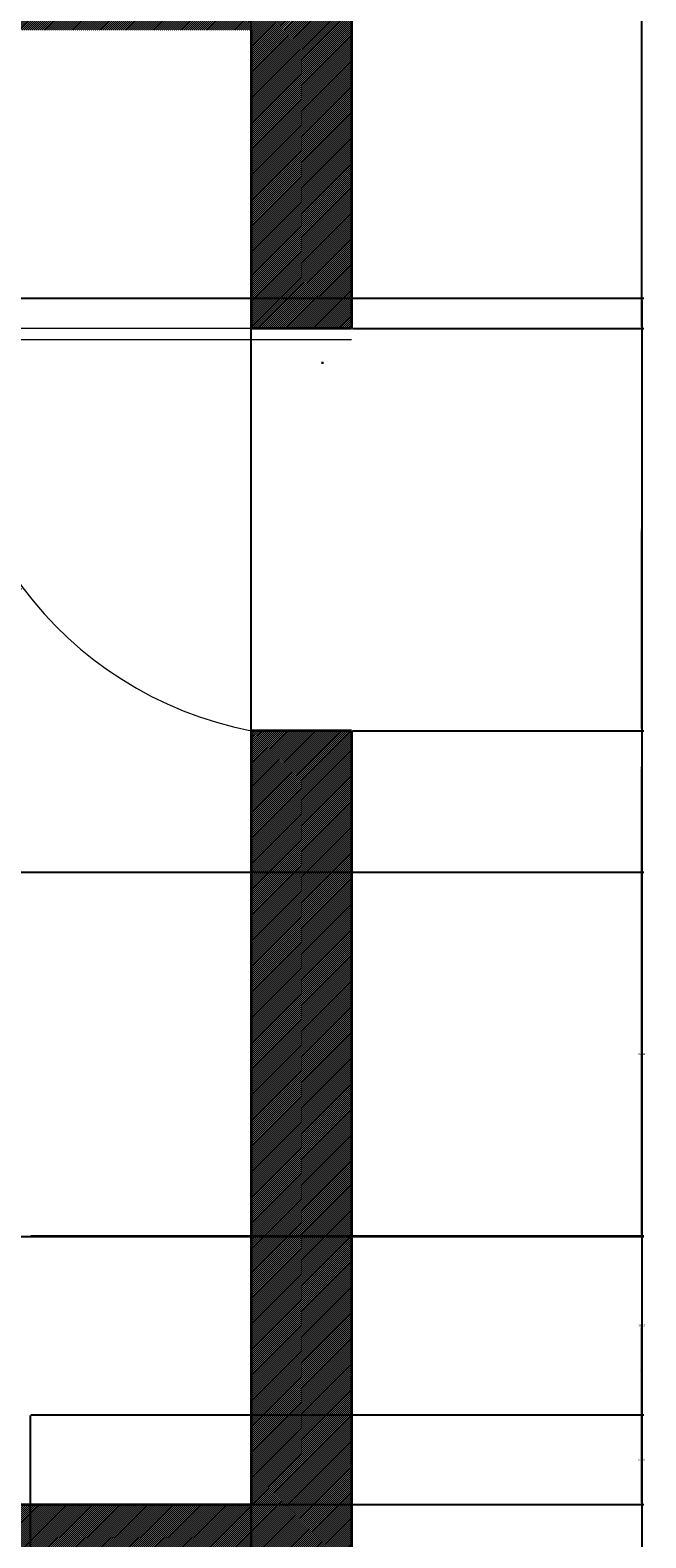
# Model space of a CAD drawing. Units: inches. Extents: x 557 to 1007, y 390 to 953.
# Tile 7 of 10: x 952 to 1007, y 612 to 747. Entities that reach past the tile are written whole.
import ezdxf

# ---------------------------------------------------------------- set-up
doc = ezdxf.new("R2010")
doc.units = ezdxf.units.IN
doc.header["$LTSCALE"] = 5
doc.header["$MEASUREMENT"] = 0
for name, color, linetype, lineweight in [('A-ANNO-DIMS', 2, 'Continuous', 18), ('A-DOOR', 3, 'Continuous', 18), ('A-WALL', 7, 'Continuous', 35)]:
    doc.layers.add(name, color=color, linetype=linetype, lineweight=lineweight)
doc.layers.add('A-WALL-PATT', color=251, linetype='Continuous', lineweight=9, true_color=0x636466)
doc.styles.get("Standard").update_dxf_attribs({"font": 'arial.ttf'})
doc.dimstyles.get("Standard").update_dxf_attribs({"dimtxt": 0.18, "dimasz": 0.18, "dimexe": 0.18, "dimexo": 0.0625, "dimgap": 0.09, "dimtad": 0, "dimtih": 1, "dimtoh": 1, "dimdec": 4, "dimzin": 0, "dimdsep": 46, "dimtxsty": 'Standard', "dimcen": 0.09, "dimadec": 0, "dimazin": 0, "dimtfac": 1, "dimtdec": 4, "dimtofl": 0, "dimtmove": 0, "dimatfit": 3, "dimfxl": 1, "dimtolj": 1, "dimtzin": 0, "dimarcsym": 0})

# ---------------------------------------------------------------- blocks, each defined once
blk = doc.blocks.new('*D55')
at = {"layer": 'A-ANNO-DIMS', "color": 0, "lineweight": -2, "ltscale": 5, "transparency": 16777216}
for p, q in [((980.47, 684.18), (1006.54, 684.18)), ((1006.36, 684), (1006.36, 562.22)), ((1006.36, 440.08), (1006.36, 561.86)), ((980.47, 439.9), (1006.54, 439.9))]:
    blk.add_line(p, q, dxfattribs=at)
at = {"layer": 'A-ANNO-DIMS', "color": 0, "ltscale": 5, "transparency": 16777216}
for points in [[(1006.33, 684), (1006.39, 684), (1006.36, 684.18)], [(1006.33, 440.08), (1006.39, 440.08), (1006.36, 439.9)]]:
    blk.add_solid(points, dxfattribs=at)
at = {"layer": 'Defpoints', "color": 0, "ltscale": 5, "transparency": 16777216}
for p in [(980.41, 684.18), (1006.36, 684.18), (980.41, 439.9)]:
    blk.add_point(p, dxfattribs=at)
at = {"layer": 'A-ANNO-DIMS', "color": 0, "ltscale": 5, "transparency": 16777216, "insert": (1006.36, 562.04), "char_height": 0.18, "attachment_point": 5}
blk.add_mtext('\\A1;244.27', dxfattribs=at)
blk = doc.blocks.new('*D56')
at = {"layer": 'A-ANNO-DIMS', "color": 0, "lineweight": -2, "ltscale": 5, "transparency": 16777216}
for p, q in [((980.47, 720.18), (1006.54, 720.18)), ((1006.36, 720), (1006.36, 702.36)), ((1006.36, 684.36), (1006.36, 702)), ((980.47, 684.18), (1006.54, 684.18))]:
    blk.add_line(p, q, dxfattribs=at)
at = {"layer": 'A-ANNO-DIMS', "color": 0, "ltscale": 5, "transparency": 16777216}
for points in [[(1006.33, 720), (1006.39, 720), (1006.36, 720.18)], [(1006.33, 684.36), (1006.39, 684.36), (1006.36, 684.18)]]:
    blk.add_solid(points, dxfattribs=at)
at = {"layer": 'Defpoints', "color": 0, "ltscale": 5, "transparency": 16777216}
for p in [(980.41, 720.18), (1006.36, 720.18), (980.41, 684.18)]:
    blk.add_point(p, dxfattribs=at)
at = {"layer": 'A-ANNO-DIMS', "color": 0, "ltscale": 5, "transparency": 16777216, "insert": (1006.36, 702.18), "char_height": 0.18, "attachment_point": 5}
blk.add_mtext('\\A1;36', dxfattribs=at)
blk = doc.blocks.new('*D57')
at = {"layer": 'A-ANNO-DIMS', "color": 0, "lineweight": -2, "ltscale": 5, "transparency": 16777216}
for p, q in [((980.47, 905.9), (1006.54, 905.9)), ((1006.36, 905.72), (1006.36, 813.22)), ((1006.36, 720.36), (1006.36, 812.86)), ((980.47, 720.18), (1006.54, 720.18))]:
    blk.add_line(p, q, dxfattribs=at)
at = {"layer": 'A-ANNO-DIMS', "color": 0, "ltscale": 5, "transparency": 16777216}
for points in [[(1006.33, 905.72), (1006.39, 905.72), (1006.36, 905.9)], [(1006.33, 720.36), (1006.39, 720.36), (1006.36, 720.18)]]:
    blk.add_solid(points, dxfattribs=at)
at = {"layer": 'Defpoints', "color": 0, "ltscale": 5, "transparency": 16777216}
for p in [(980.41, 905.9), (1006.36, 905.9), (980.41, 720.18)]:
    blk.add_point(p, dxfattribs=at)
at = {"layer": 'A-ANNO-DIMS', "color": 0, "ltscale": 5, "transparency": 16777216, "insert": (1006.36, 813.04), "char_height": 0.18, "attachment_point": 5}
blk.add_mtext('\\A1;185.73', dxfattribs=at)
blk = doc.blocks.new('*D60')
at = {"layer": 'A-ANNO-DIMS', "color": 0, "lineweight": -2, "ltscale": 5, "transparency": 16777216}
for p, q in [((683.47, 722.9), (1006.54, 722.9)), ((1006.36, 722.72), (1006.36, 681.09)), ((1006.36, 639.08), (1006.36, 680.72)), ((683.47, 638.9), (1006.54, 638.9))]:
    blk.add_line(p, q, dxfattribs=at)
at = {"layer": 'A-ANNO-DIMS', "color": 0, "ltscale": 5, "transparency": 16777216}
for points in [[(1006.33, 722.72), (1006.39, 722.72), (1006.36, 722.9)], [(1006.33, 639.08), (1006.39, 639.08), (1006.36, 638.9)]]:
    blk.add_solid(points, dxfattribs=at)
at = {"layer": 'Defpoints', "color": 0, "ltscale": 5, "transparency": 16777216}
for p in [(683.41, 722.9), (683.41, 638.9), (1006.36, 638.9)]:
    blk.add_point(p, dxfattribs=at)
at = {"layer": 'A-ANNO-DIMS', "color": 0, "ltscale": 5, "transparency": 16777216, "insert": (1006.36, 680.9), "char_height": 0.18, "attachment_point": 5}
blk.add_mtext('\\A1;84', dxfattribs=at)
blk = doc.blocks.new('*D61')
at = {"layer": 'A-ANNO-DIMS', "color": 0, "lineweight": -2, "ltscale": 5, "transparency": 16777216}
for p, q in [((683.47, 638.9), (1006.54, 638.9)), ((1006.36, 638.72), (1006.36, 627.08)), ((1006.36, 615.08), (1006.36, 626.72)), ((683.47, 614.9), (1006.54, 614.9))]:
    blk.add_line(p, q, dxfattribs=at)
at = {"layer": 'A-ANNO-DIMS', "color": 0, "ltscale": 5, "transparency": 16777216}
for points in [[(1006.33, 638.72), (1006.39, 638.72), (1006.36, 638.9)], [(1006.33, 615.08), (1006.39, 615.08), (1006.36, 614.9)]]:
    blk.add_solid(points, dxfattribs=at)
at = {"layer": 'Defpoints', "color": 0, "ltscale": 5, "transparency": 16777216}
for p in [(683.41, 638.9), (683.41, 614.9), (1006.36, 614.9)]:
    blk.add_point(p, dxfattribs=at)
at = {"layer": 'A-ANNO-DIMS', "color": 0, "ltscale": 5, "transparency": 16777216, "insert": (1006.36, 626.9), "char_height": 0.18, "attachment_point": 5}
blk.add_mtext('\\A1;24', dxfattribs=at)
blk = doc.blocks.new('*D85')
at = {"layer": 'A-ANNO-DIMS', "color": 0, "lineweight": -2, "ltscale": 5, "transparency": 16777216}
for p, q in [((951.7, 638.94), (1006.54, 638.94)), ((1006.36, 638.76), (1006.36, 631.11)), ((1006.36, 623.1), (1006.36, 630.75)), ((951.7, 622.92), (1006.54, 622.92))]:
    blk.add_line(p, q, dxfattribs=at)
at = {"layer": 'A-ANNO-DIMS', "color": 0, "ltscale": 5, "transparency": 16777216}
for points in [[(1006.33, 638.76), (1006.39, 638.76), (1006.36, 638.94)], [(1006.33, 623.1), (1006.39, 623.1), (1006.36, 622.92)]]:
    blk.add_solid(points, dxfattribs=at)
at = {"layer": 'Defpoints', "color": 0, "ltscale": 5, "transparency": 16777216}
for p in [(951.64, 638.94), (1006.36, 638.94), (951.64, 622.92)]:
    blk.add_point(p, dxfattribs=at)
at = {"layer": 'A-ANNO-DIMS', "color": 0, "ltscale": 5, "transparency": 16777216, "insert": (1006.36, 630.93), "char_height": 0.18, "attachment_point": 5}
blk.add_mtext('\\A1;16.02', dxfattribs=at)
blk = doc.blocks.new('*D88')
at = {"layer": 'A-ANNO-DIMS', "color": 0, "lineweight": -2, "ltscale": 5, "transparency": 16777216}
for p, q in [((944.01, 671.52), (1006.54, 671.52)), ((1006.36, 671.34), (1006.36, 655.41)), ((1006.36, 639.12), (1006.36, 655.05)), ((951.7, 638.94), (1006.54, 638.94))]:
    blk.add_line(p, q, dxfattribs=at)
at = {"layer": 'A-ANNO-DIMS', "color": 0, "ltscale": 5, "transparency": 16777216}
for points in [[(1006.33, 671.34), (1006.39, 671.34), (1006.36, 671.52)], [(1006.33, 639.12), (1006.39, 639.12), (1006.36, 638.94)]]:
    blk.add_solid(points, dxfattribs=at)
at = {"layer": 'Defpoints', "color": 0, "ltscale": 5, "transparency": 16777216}
for p in [(943.95, 671.52), (951.64, 638.94), (1006.36, 638.94)]:
    blk.add_point(p, dxfattribs=at)
at = {"layer": 'A-ANNO-DIMS', "color": 0, "ltscale": 5, "transparency": 16777216, "insert": (1006.36, 655.23), "char_height": 0.18, "attachment_point": 5}
blk.add_mtext('\\A1;32.58', dxfattribs=at)
blk = doc.blocks.new('*D89')
at = {"layer": 'A-ANNO-DIMS', "color": 0, "lineweight": -2, "ltscale": 5, "transparency": 16777216}
for p, q in [((951.64, 622.86), (951.64, 389.77)), ((971.41, 614.84), (971.41, 389.77)), ((951.82, 389.95), (961.07, 389.95)), ((971.23, 389.95), (961.98, 389.95))]:
    blk.add_line(p, q, dxfattribs=at)
at = {"layer": 'A-ANNO-DIMS', "color": 0, "ltscale": 5, "transparency": 16777216}
for points in [[(951.82, 389.98), (951.82, 389.92), (951.64, 389.95)], [(971.23, 389.98), (971.23, 389.92), (971.41, 389.95)]]:
    blk.add_solid(points, dxfattribs=at)
at = {"layer": 'Defpoints', "color": 0, "ltscale": 5, "transparency": 16777216}
for p in [(951.64, 622.92), (971.41, 614.9), (971.41, 389.95)]:
    blk.add_point(p, dxfattribs=at)
at = {"layer": 'A-ANNO-DIMS', "color": 0, "ltscale": 5, "transparency": 16777216, "insert": (961.52, 389.95), "char_height": 0.18, "attachment_point": 5}
blk.add_mtext('\\A1;19.765', dxfattribs=at)
blk = doc.blocks.new('*D90')
at = {"layer": 'A-ANNO-DIMS', "color": 0, "lineweight": -2, "ltscale": 5, "transparency": 16777216}
for p, q in [((951.7, 622.92), (1006.54, 622.92)), ((1006.36, 622.74), (1006.36, 619.1)), ((1006.36, 615.08), (1006.36, 618.73)), ((971.47, 614.9), (1006.54, 614.9))]:
    blk.add_line(p, q, dxfattribs=at)
at = {"layer": 'A-ANNO-DIMS', "color": 0, "ltscale": 5, "transparency": 16777216}
for points in [[(1006.33, 622.74), (1006.39, 622.74), (1006.36, 622.92)], [(1006.33, 615.08), (1006.39, 615.08), (1006.36, 614.9)]]:
    blk.add_solid(points, dxfattribs=at)
at = {"layer": 'Defpoints', "color": 0, "ltscale": 5, "transparency": 16777216}
for p in [(951.64, 622.92), (1006.36, 622.92), (971.41, 614.9)]:
    blk.add_point(p, dxfattribs=at)
at = {"layer": 'A-ANNO-DIMS', "color": 0, "ltscale": 5, "transparency": 16777216, "insert": (1006.36, 618.91), "char_height": 0.18, "attachment_point": 5}
blk.add_mtext('\\A1;8.019', dxfattribs=at)
blk = doc.blocks.new('*D96')
at = {"layer": 'A-ANNO-DIMS', "color": 0, "lineweight": -2, "ltscale": 5, "transparency": 16777216}
for p, q in [((947.41, 536.97), (947.41, 953.03)), ((947.59, 952.85), (959.19, 952.85)), ((971.23, 952.85), (959.63, 952.85)), ((971.41, 512.97), (971.41, 953.03))]:
    blk.add_line(p, q, dxfattribs=at)
at = {"layer": 'A-ANNO-DIMS', "color": 0, "ltscale": 5, "transparency": 16777216}
for points in [[(947.59, 952.88), (947.59, 952.82), (947.41, 952.85)], [(971.23, 952.88), (971.23, 952.82), (971.41, 952.85)]]:
    blk.add_solid(points, dxfattribs=at)
at = {"layer": 'Defpoints', "color": 0, "ltscale": 5, "transparency": 16777216}
for p in [(971.41, 952.85), (947.41, 536.9), (971.41, 512.9)]:
    blk.add_point(p, dxfattribs=at)
at = {"layer": 'A-ANNO-DIMS', "color": 0, "ltscale": 5, "transparency": 16777216, "insert": (959.41, 952.85), "char_height": 0.18, "attachment_point": 5}
blk.add_mtext('\\A1;24', dxfattribs=at)
blk = doc.blocks.new('*D105')
at = {"layer": 'A-ANNO-DIMS', "color": 0, "lineweight": -2, "ltscale": 5, "transparency": 16777216}
for p, q in [((977.72, 717.11), (977.9, 717.11)), ((977.81, 717.02), (977.81, 717.2)), ((934.87, 684.9), (950.83, 696.87)), ((934.69, 684.9), (934.87, 684.9))]:
    blk.add_line(p, q, dxfattribs=at)
at = {"layer": 'A-ANNO-DIMS', "color": 0, "ltscale": 5, "transparency": 16777216}
blk.add_solid([(950.81, 696.9), (950.85, 696.85), (950.97, 696.98)], dxfattribs=at)
at = {"layer": 'Defpoints', "color": 0, "ltscale": 5, "transparency": 16777216}
for p in [(977.81, 717.11), (950.97, 696.98)]:
    blk.add_point(p, dxfattribs=at)
at = {"layer": 'A-ANNO-DIMS', "color": 0, "ltscale": 5, "transparency": 16777216, "insert": (934.14, 684.9), "char_height": 0.18, "attachment_point": 5}
blk.add_mtext('\\A1;R33.545', dxfattribs=at)

msp = doc.modelspace()

# ---------------------------------------------------------------- hatches: boundary and pattern name
at = {"layer": 'A-WALL-PATT'}
h = msp.add_hatch(dxfattribs=at)
h.set_pattern_fill('ANSI31', color=256)
h.paths.add_polyline_path([(808.0625, 905.9046), (767.4053, 905.9046), (767.4053, 920.9046), (839.4053, 920.9046), (839.4053, 905.9046), (832.0625, 905.9046), (832.0625, 896.9046), (839.4053, 896.9046), (839.4053, 800.9046), (837.4053, 800.9046), (837.4053, 794.9046), (839.4053, 794.9046), (839.4053, 790.9046), (845.4053, 790.9046), (845.4053, 896.9046), (878.4053, 896.9046), (878.4053, 905.9046), (845.4053, 905.9046), (845.4053, 926.9046), (761.4053, 926.9046), (761.4053, 914.9046), (761.4053, 905.9046), (724.9087, 905.9046), (724.9087, 896.9046), (761.4053, 896.9046), (761.4053, 752.9046), (759.4053, 752.9046), (759.4053, 746.9046), (767.4053, 746.9046), (767.4053, 794.9046), (807.4053, 794.9046), (807.4053, 800.9046), (767.4053, 800.9046), (767.4053, 896.9046), (808.0625, 896.9046)])
h.paths.add_polyline_path([(676.9087, 905.9046), (632.4053, 905.9046), (632.4053, 838.7688), (641.4053, 838.7688), (641.4053, 881.8539), (641.4053, 896.9046), (676.9087, 896.9046)])
h.paths.add_polyline_path([(980.4053, 905.9046), (938.4053, 905.9046), (938.4053, 896.9046), (971.4053, 896.9046), (971.4053, 752.9046), (845.4053, 752.9046), (845.4053, 754.9046), (839.4053, 754.9046), (839.4053, 746.9046), (971.4053, 746.9046), (971.4053, 720.1788), (980.4053, 720.1788)])
h.paths.add_polyline_path([(723.4053, 752.9046), (641.4053, 752.9046), (641.4053, 790.7688), (632.4053, 790.7688), (632.4053, 743.9046), (674.4053, 743.9046), (674.4053, 722.9046), (683.4053, 722.9046), (683.4053, 746.9046), (723.4053, 746.9046)])
h.paths.add_polyline_path([(980.4053, 684.1788), (971.4053, 684.1788), (971.4053, 614.9046), (845.4053, 614.9046), (845.4053, 608.9046), (971.4053, 608.9046), (971.4053, 512.9046), (908.7697, 512.9046), (908.7697, 508.9046), (971.4053, 508.9046), (971.4053, 448.9046), (845.4053, 448.9046), (845.4053, 508.9046), (878.7697, 508.9046), (878.7697, 512.9046), (845.4053, 512.9046), (845.4053, 562.9046), (779.4053, 562.9046), (779.4053, 614.9046), (761.4053, 614.9046), (761.4053, 608.9046), (773.4053, 608.9046), (773.4053, 512.636), (779.4053, 512.636), (779.4053, 556.9046), (839.4053, 556.9046), (839.4053, 448.9046), (830.432, 448.9046), (830.432, 439.9046), (839.4053, 439.9046), (839.4053, 433.0506), (839.4053, 421.9046), (779.4053, 421.9046), (779.4053, 439.9046), (796.9656, 439.9046), (806.432, 439.9046), (806.432, 448.9046), (779.4053, 448.9046), (779.4053, 482.636), (773.4053, 482.636), (773.4053, 448.9046), (764.9579, 448.9046), (764.9579, 439.9046), (773.4053, 439.9046), (773.4053, 415.9046), (845.4053, 415.9046), (845.4053, 439.9046), (980.4053, 439.9046)])
h.paths.add_polyline_path([(716.9579, 448.9046), (641.4053, 448.9046), (641.4053, 557.9046), (632.4053, 557.9046), (632.4053, 439.9046), (716.9579, 439.9046)])
h.paths.add_polyline_path([(725.4053, 614.9046), (683.4053, 614.9046), (683.4053, 638.9046), (674.4053, 638.9046), (674.4053, 614.9046), (608.4053, 614.9046), (582.8236, 614.9046), (582.8236, 605.9046), (599.4053, 605.9046), (632.4053, 605.9046), (641.4053, 605.9046), (641.4053, 608.9046), (725.4053, 608.9046)])
h.paths.add_polyline_path([(641.4053, 605.9046), (632.4053, 605.9046), (632.4053, 593.9046), (641.4053, 593.9046)])

# ---------------------------------------------------------------- linework, layer by layer
at = {"layer": 'A-DOOR'}
for p, q in [((980.4053, 720.1788), (944.4053, 720.1788)), ((980.4053, 719.1788), (944.4053, 719.1788))]:
    msp.add_line(p, q, dxfattribs=at)
msp.add_arc((977.809, 717.1066), 33.5447, 174.745153, 258.994642, dxfattribs=at)
at = {"layer": 'A-WALL'}
for p, q in [((980.4053, 905.9046), (980.4053, 720.1788)), ((971.4053, 746.9046), (971.4053, 720.1788)), ((980.4053, 720.1788), (971.4053, 720.1788)), ((980.4053, 684.1788), (971.4053, 684.1788)), ((971.4053, 684.1788), (971.4053, 614.9046)), ((980.4053, 684.1788), (980.4053, 439.9046)), ((845.4053, 614.9046), (971.4053, 614.9046))]:
    msp.add_line(p, q, dxfattribs=at)

# ---------------------------------------------------------------- dimensions: what is measured, and where the dimension line sits
at = {"layer": 'A-ANNO-DIMS', "ltscale": 5}
for base, p1, p2, override, picture, middle in [((971.4053, 952.8546), (947.4053, 536.9046), (971.4053, 512.9046), {"dimdec": 0, "dimlfac": 1, "dimrnd": 0, "dimzin": 0, "dimdsep": 46, "dimlunit": 2}, '*D96', (959.4053, 952.8546)), ((971.4053, 389.9546), (951.6399, 622.9231), (971.4053, 614.9046), {"dimdec": 3, "dimlfac": 1, "dimrnd": 0, "dimzin": 0, "dimdsep": 46, "dimlunit": 2}, '*D89', (961.5226, 389.9546))]:
    dim = msp.add_linear_dim(base=base, p1=p1, p2=p2, dimstyle='Standard', override=override, dxfattribs=at)
    dim.commit()
    dim.dimension.update_dxf_attribs({"geometry": picture, "text_midpoint": middle})
for base, p1, p2, override, picture, middle in [((1006.3553, 905.9046), (980.4053, 720.1788), (980.4053, 905.9046), {"dimdec": 2, "dimlfac": 1, "dimrnd": 0, "dimzin": 0, "dimdsep": 46, "dimlunit": 2}, '*D57', (1006.3553, 813.0417)), ((1006.3553, 638.9046), (683.4053, 722.9046), (683.4053, 638.9046), {"dimdec": 0, "dimlfac": 1, "dimrnd": 0, "dimzin": 0, "dimdsep": 46, "dimlunit": 2}, '*D60', (1006.3553, 680.9046)), ((1006.3553, 720.1788), (980.4053, 684.1788), (980.4053, 720.1788), {"dimdec": 0, "dimlfac": 1, "dimrnd": 0, "dimzin": 0, "dimdsep": 46, "dimlunit": 2}, '*D56', (1006.3553, 702.1788)), ((1006.3553, 684.1788), (980.4053, 439.9046), (980.4053, 684.1788), {"dimdec": 2, "dimlfac": 1, "dimrnd": 0, "dimzin": 0, "dimdsep": 46, "dimlunit": 2}, '*D55', (1006.3553, 562.0417)), ((1006.3553, 638.9424), (943.9465, 671.5202), (951.6399, 638.9424), {"dimdec": 2, "dimlfac": 1, "dimrnd": 0, "dimzin": 0, "dimdsep": 46, "dimlunit": 2}, '*D88', (1006.3553, 655.2313)), ((1006.3553, 614.9046), (683.4053, 638.9046), (683.4053, 614.9046), {"dimdec": 0, "dimlfac": 1, "dimrnd": 0, "dimzin": 0, "dimdsep": 46, "dimlunit": 2}, '*D61', (1006.3553, 626.9046)), ((1006.3553, 638.9424), (951.6399, 622.9231), (951.6399, 638.9424), {"dimdec": 2, "dimlfac": 1, "dimrnd": 0, "dimzin": 0, "dimdsep": 46, "dimlunit": 2}, '*D85', (1006.3553, 630.9328)), ((1006.35526, 622.9231), (971.40526, 614.90457), (951.63986, 622.9231), {"dimdec": 3, "dimlfac": 1, "dimrnd": 0, "dimzin": 0, "dimdsep": 46, "dimlunit": 2}, '*D90', (1006.35526, 618.91383))]:
    dim = msp.add_linear_dim(base=base, p1=p1, p2=p2, angle=90, dimstyle='Standard', override=override, dxfattribs=at)
    dim.commit()
    dim.dimension.update_dxf_attribs({"geometry": picture, "text_midpoint": middle})
dim = msp.add_radius_dim(center=(977.809, 717.1066), mpoint=(950.973, 696.98), dimstyle='Standard', override={"dimdec": 3, "dimlfac": 1, "dimrnd": 0, "dimzin": 0, "dimdsep": 46, "dimlunit": 2}, dxfattribs=at)
dim.commit()
dim.dimension.update_dxf_attribs({"geometry": '*D105', "text_midpoint": (934.1411, 684.9041), "dimtype": 164})

doc.saveas('drawing.dxf')
